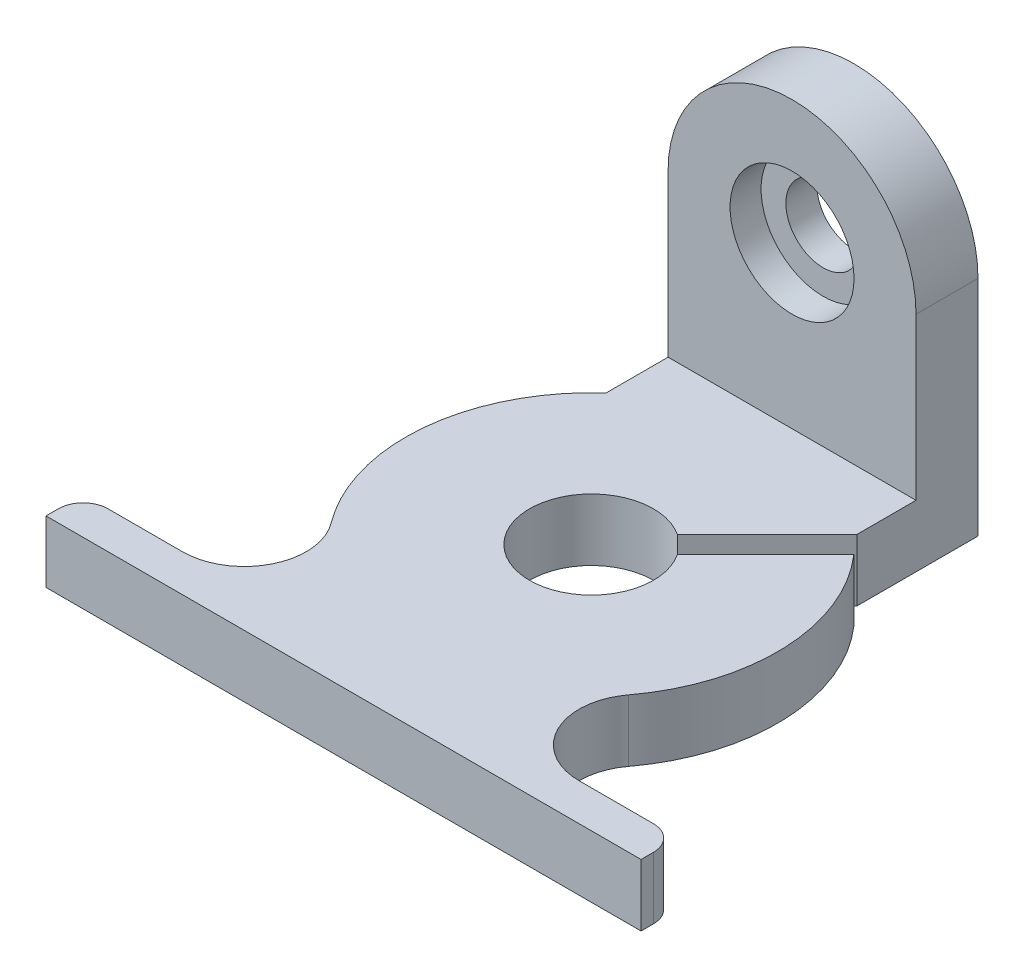
ISO-10303-21;
HEADER;
FILE_DESCRIPTION(('STEP AP214'),'2;1');
FILE_NAME('part.step','',(''),(''),'','','');
FILE_SCHEMA(('AUTOMOTIVE_DESIGN { 1 0 10303 214 1 1 1 1 }'));
ENDSEC;
DATA;
#1=APPLICATION_CONTEXT('core data for automotive mechanical design processes');
#2=APPLICATION_PROTOCOL_DEFINITION('international standard','automotive_design',2000,#1);
#3=PRODUCT_CONTEXT('',#1,'mechanical');
#4=PRODUCT('Part','Part','',(#3));
#5=PRODUCT_RELATED_PRODUCT_CATEGORY('part','',(#4));
#6=PRODUCT_DEFINITION_FORMATION('','',#4);
#7=PRODUCT_DEFINITION_CONTEXT('part definition',#1,'design');
#8=PRODUCT_DEFINITION('design','',#6,#7);
#9=PRODUCT_DEFINITION_SHAPE('','',#8);
#10=(LENGTH_UNIT() NAMED_UNIT(*) SI_UNIT(.MILLI.,.METRE.));
#11=(NAMED_UNIT(*) PLANE_ANGLE_UNIT() SI_UNIT($,.RADIAN.));
#12=(NAMED_UNIT(*) SI_UNIT($,.STERADIAN.) SOLID_ANGLE_UNIT());
#13=UNCERTAINTY_MEASURE_WITH_UNIT(LENGTH_MEASURE(1.E-05),#10,'distance_accuracy_value','');
#14=(GEOMETRIC_REPRESENTATION_CONTEXT(3) GLOBAL_UNCERTAINTY_ASSIGNED_CONTEXT((#13)) GLOBAL_UNIT_ASSIGNED_CONTEXT((#10,
#11,#12)) REPRESENTATION_CONTEXT('',''));
#15=CARTESIAN_POINT('',(0.,0.,0.));
#16=DIRECTION('',(0.,0.,1.));
#17=DIRECTION('',(1.,0.,0.));
#18=AXIS2_PLACEMENT_3D('',#15,#16,#17);
#19=CARTESIAN_POINT('',(0.,18.,-36.180339887499));
#20=DIRECTION('',(0.,0.,-1.));
#21=DIRECTION('',(-1.,0.,0.));
#22=AXIS2_PLACEMENT_3D('',#19,#20,#21);
#23=CYLINDRICAL_SURFACE('',#22,3.);
#24=CARTESIAN_POINT('',(0.,18.,-41.180339887499));
#25=DIRECTION('',(0.,0.,-1.));
#26=DIRECTION('',(-1.,0.,0.));
#27=AXIS2_PLACEMENT_3D('',#24,#25,#26);
#28=CIRCLE('',#27,3.);
#29=CARTESIAN_POINT('',(-3.,18.,-41.180339887499));
#30=VERTEX_POINT('',#29);
#31=EDGE_CURVE('E596',#30,#30,#28,.T.);
#32=ORIENTED_EDGE('',*,*,#31,.T.);
#33=EDGE_LOOP('',(#32));
#34=FACE_BOUND('',#33,.T.);
#35=CARTESIAN_POINT('',(0.,18.,-38.680339887499));
#36=DIRECTION('',(0.,0.,1.));
#37=DIRECTION('',(1.,0.,0.));
#38=AXIS2_PLACEMENT_3D('',#35,#36,#37);
#39=CIRCLE('',#38,3.);
#40=CARTESIAN_POINT('',(3.,18.,-38.680339887499));
#41=VERTEX_POINT('',#40);
#42=EDGE_CURVE('E609',#41,#41,#39,.T.);
#43=ORIENTED_EDGE('',*,*,#42,.T.);
#44=EDGE_LOOP('',(#43));
#45=FACE_BOUND('',#44,.T.);
#46=ADVANCED_FACE('F50',(#34,#45),#23,.F.);
#47=CARTESIAN_POINT('',(0.,5.,0.));
#48=DIRECTION('',(0.,1.,0.));
#49=DIRECTION('',(0.,0.,1.));
#50=AXIS2_PLACEMENT_3D('',#47,#48,#49);
#51=PLANE('',#50);
#52=DIRECTION('',(0.,0.,-1.));
#53=VECTOR('',#52,1.);
#54=CARTESIAN_POINT('',(10.,5.,0.));
#55=LINE('',#54,#53);
#56=CARTESIAN_POINT('',(10.,5.,-31.4142135623731));
#57=VERTEX_POINT('',#56);
#58=CARTESIAN_POINT('',(10.,5.,-36.180339887499));
#59=VERTEX_POINT('',#58);
#60=EDGE_CURVE('E197',#57,#59,#55,.T.);
#61=ORIENTED_EDGE('',*,*,#60,.T.);
#62=DIRECTION('',(-1.,0.,0.));
#63=VECTOR('',#62,1.);
#64=CARTESIAN_POINT('',(0.,5.,-36.180339887499));
#65=LINE('',#64,#63);
#66=CARTESIAN_POINT('',(-10.,5.,-36.180339887499));
#67=VERTEX_POINT('',#66);
#68=EDGE_CURVE('E202',#59,#67,#65,.T.);
#69=ORIENTED_EDGE('',*,*,#68,.T.);
#70=DIRECTION('',(0.,0.,-1.));
#71=VECTOR('',#70,1.);
#72=CARTESIAN_POINT('',(-10.,5.,0.));
#73=LINE('',#72,#71);
#74=CARTESIAN_POINT('',(-10.,5.,-31.1803398874989));
#75=VERTEX_POINT('',#74);
#76=EDGE_CURVE('E241',#75,#67,#73,.T.);
#77=ORIENTED_EDGE('',*,*,#76,.F.);
#78=CARTESIAN_POINT('',(0.,5.,-20.));
#79=DIRECTION('',(0.,1.,0.));
#80=DIRECTION('',(0.,0.,1.));
#81=AXIS2_PLACEMENT_3D('',#78,#79,#80);
#82=CIRCLE('',#81,15.);
#83=CARTESIAN_POINT('',(-12.,5.,-11.));
#84=VERTEX_POINT('',#83);
#85=EDGE_CURVE('E291',#75,#84,#82,.T.);
#86=ORIENTED_EDGE('',*,*,#85,.T.);
#87=CARTESIAN_POINT('',(-16.,5.,-8.));
#88=DIRECTION('',(0.,1.,0.));
#89=DIRECTION('',(0.,0.,1.));
#90=AXIS2_PLACEMENT_3D('',#87,#88,#89);
#91=CIRCLE('',#90,5.);
#92=CARTESIAN_POINT('',(-16.,5.,-3.));
#93=VERTEX_POINT('',#92);
#94=EDGE_CURVE('E280',#84,#93,#91,.F.);
#95=ORIENTED_EDGE('',*,*,#94,.T.);
#96=DIRECTION('',(1.,0.,0.));
#97=VECTOR('',#96,1.);
#98=CARTESIAN_POINT('',(0.,5.,-3.));
#99=LINE('',#98,#97);
#100=CARTESIAN_POINT('',(-22.,5.,-3.));
#101=VERTEX_POINT('',#100);
#102=EDGE_CURVE('E288',#101,#93,#99,.T.);
#103=ORIENTED_EDGE('',*,*,#102,.F.);
#104=CARTESIAN_POINT('',(-22.,5.,-1.));
#105=DIRECTION('',(0.,1.,0.));
#106=DIRECTION('',(0.,0.,1.));
#107=AXIS2_PLACEMENT_3D('',#104,#105,#106);
#108=CIRCLE('',#107,2.);
#109=CARTESIAN_POINT('',(-24.,5.,-0.999999999999985));
#110=VERTEX_POINT('',#109);
#111=EDGE_CURVE('E290',#110,#101,#108,.F.);
#112=ORIENTED_EDGE('',*,*,#111,.F.);
#113=DIRECTION('',(0.,0.,-1.));
#114=VECTOR('',#113,1.);
#115=CARTESIAN_POINT('',(-24.,5.,0.));
#116=LINE('',#115,#114);
#117=CARTESIAN_POINT('',(-24.,5.,0.));
#118=VERTEX_POINT('',#117);
#119=EDGE_CURVE('E292',#118,#110,#116,.T.);
#120=ORIENTED_EDGE('',*,*,#119,.F.);
#121=DIRECTION('',(1.,0.,0.));
#122=VECTOR('',#121,1.);
#123=CARTESIAN_POINT('',(0.,5.,0.));
#124=LINE('',#123,#122);
#125=CARTESIAN_POINT('',(24.,5.,0.));
#126=VERTEX_POINT('',#125);
#127=EDGE_CURVE('E300',#118,#126,#124,.T.);
#128=ORIENTED_EDGE('',*,*,#127,.T.);
#129=DIRECTION('',(0.,0.,1.));
#130=VECTOR('',#129,1.);
#131=CARTESIAN_POINT('',(24.,5.,0.));
#132=LINE('',#131,#130);
#133=CARTESIAN_POINT('',(24.,5.,-0.999999999999985));
#134=VERTEX_POINT('',#133);
#135=EDGE_CURVE('E303',#134,#126,#132,.T.);
#136=ORIENTED_EDGE('',*,*,#135,.F.);
#137=CARTESIAN_POINT('',(22.,5.,-1.));
#138=DIRECTION('',(0.,1.,0.));
#139=DIRECTION('',(0.,0.,1.));
#140=AXIS2_PLACEMENT_3D('',#137,#138,#139);
#141=CIRCLE('',#140,2.);
#142=CARTESIAN_POINT('',(22.,5.,-3.));
#143=VERTEX_POINT('',#142);
#144=EDGE_CURVE('E305',#143,#134,#141,.F.);
#145=ORIENTED_EDGE('',*,*,#144,.F.);
#146=DIRECTION('',(1.,0.,0.));
#147=VECTOR('',#146,1.);
#148=CARTESIAN_POINT('',(0.,5.,-3.));
#149=LINE('',#148,#147);
#150=CARTESIAN_POINT('',(16.,5.,-3.));
#151=VERTEX_POINT('',#150);
#152=EDGE_CURVE('E307',#151,#143,#149,.T.);
#153=ORIENTED_EDGE('',*,*,#152,.F.);
#154=CARTESIAN_POINT('',(16.,5.,-8.));
#155=DIRECTION('',(0.,1.,0.));
#156=DIRECTION('',(0.,0.,1.));
#157=AXIS2_PLACEMENT_3D('',#154,#155,#156);
#158=CIRCLE('',#157,5.);
#159=CARTESIAN_POINT('',(12.,5.,-11.));
#160=VERTEX_POINT('',#159);
#161=EDGE_CURVE('E309',#160,#151,#158,.T.);
#162=ORIENTED_EDGE('',*,*,#161,.F.);
#163=CARTESIAN_POINT('',(0.,5.,-20.));
#164=DIRECTION('',(0.,1.,0.));
#165=DIRECTION('',(0.,0.,1.));
#166=AXIS2_PLACEMENT_3D('',#163,#164,#165);
#167=CIRCLE('',#166,15.);
#168=CARTESIAN_POINT('',(11.2901120254449,5.,-29.8758984630718));
#169=VERTEX_POINT('',#168);
#170=EDGE_CURVE('E194',#160,#169,#167,.T.);
#171=ORIENTED_EDGE('',*,*,#170,.T.);
#172=DIRECTION('',(0.707106781186549,0.,-0.707106781186546));
#173=VECTOR('',#172,1.);
#174=CARTESIAN_POINT('',(-9.29289321881346,5.,-9.29289321881349));
#175=LINE('',#174,#173);
#176=CARTESIAN_POINT('',(4.17120839632431,5.,-22.7569948339512));
#177=VERTEX_POINT('',#176);
#178=EDGE_CURVE('E177',#177,#169,#175,.T.);
#179=ORIENTED_EDGE('',*,*,#178,.F.);
#180=CARTESIAN_POINT('',(0.,5.,-20.));
#181=DIRECTION('',(0.,1.,0.));
#182=DIRECTION('',(0.,0.,1.));
#183=AXIS2_PLACEMENT_3D('',#180,#181,#182);
#184=CIRCLE('',#183,5.);
#185=CARTESIAN_POINT('',(2.75699483395122,5.,-24.1712083963243));
#186=VERTEX_POINT('',#185);
#187=EDGE_CURVE('E190',#186,#177,#184,.T.);
#188=ORIENTED_EDGE('',*,*,#187,.F.);
#189=DIRECTION('',(0.707106781186549,0.,-0.707106781186547));
#190=VECTOR('',#189,1.);
#191=CARTESIAN_POINT('',(-10.7071067811865,5.,-10.7071067811866));
#192=LINE('',#191,#190);
#193=EDGE_CURVE('E65',#186,#57,#192,.T.);
#194=ORIENTED_EDGE('',*,*,#193,.T.);
#195=EDGE_LOOP('',(#61,#69,#77,#86,#95,#103,#112,#120,#128,#136,#145,#153,#162,#171,#179,#188,#194));
#196=FACE_BOUND('',#195,.T.);
#197=ADVANCED_FACE('F187',(#196),#51,.T.);
#198=CARTESIAN_POINT('',(-10.,5.,0.));
#199=DIRECTION('',(-1.,0.,0.));
#200=DIRECTION('',(0.,0.,1.));
#201=AXIS2_PLACEMENT_3D('',#198,#199,#200);
#202=PLANE('',#201);
#203=DIRECTION('',(0.,-1.,0.));
#204=VECTOR('',#203,1.);
#205=CARTESIAN_POINT('',(-10.,5.,-41.180339887499));
#206=LINE('',#205,#204);
#207=CARTESIAN_POINT('',(-10.,18.,-41.180339887499));
#208=VERTEX_POINT('',#207);
#209=CARTESIAN_POINT('',(-10.,0.,-41.180339887499));
#210=VERTEX_POINT('',#209);
#211=EDGE_CURVE('E205',#208,#210,#206,.T.);
#212=ORIENTED_EDGE('',*,*,#211,.T.);
#213=DIRECTION('',(0.,0.,-1.));
#214=VECTOR('',#213,1.);
#215=CARTESIAN_POINT('',(-10.,0.,0.));
#216=LINE('',#215,#214);
#217=CARTESIAN_POINT('',(-10.,0.,-31.1803398874989));
#218=VERTEX_POINT('',#217);
#219=EDGE_CURVE('E129',#218,#210,#216,.T.);
#220=ORIENTED_EDGE('',*,*,#219,.F.);
#221=DIRECTION('',(0.,-1.,0.));
#222=VECTOR('',#221,1.);
#223=CARTESIAN_POINT('',(-10.,5.,-31.1803398874989));
#224=LINE('',#223,#222);
#225=EDGE_CURVE('E11',#75,#218,#224,.T.);
#226=ORIENTED_EDGE('',*,*,#225,.F.);
#227=ORIENTED_EDGE('',*,*,#76,.T.);
#228=DIRECTION('',(0.,1.,0.));
#229=VECTOR('',#228,1.);
#230=CARTESIAN_POINT('',(-10.,0.,-36.180339887499));
#231=LINE('',#230,#229);
#232=CARTESIAN_POINT('',(-10.,18.,-36.180339887499));
#233=VERTEX_POINT('',#232);
#234=EDGE_CURVE('E589',#67,#233,#231,.T.);
#235=ORIENTED_EDGE('',*,*,#234,.T.);
#236=DIRECTION('',(0.,0.,-1.));
#237=VECTOR('',#236,1.);
#238=CARTESIAN_POINT('',(-10.,18.,-36.180339887499));
#239=LINE('',#238,#237);
#240=EDGE_CURVE('E584',#233,#208,#239,.T.);
#241=ORIENTED_EDGE('',*,*,#240,.T.);
#242=EDGE_LOOP('',(#212,#220,#226,#227,#235,#241));
#243=FACE_BOUND('',#242,.T.);
#244=ADVANCED_FACE('F47',(#243),#202,.T.);
#245=CARTESIAN_POINT('',(0.,5.,-20.));
#246=DIRECTION('',(0.,-1.,0.));
#247=DIRECTION('',(0.,0.,-1.));
#248=AXIS2_PLACEMENT_3D('',#245,#246,#247);
#249=CYLINDRICAL_SURFACE('',#248,15.);
#250=CARTESIAN_POINT('',(0.,0.,-20.));
#251=DIRECTION('',(0.,1.,0.));
#252=DIRECTION('',(0.,0.,1.));
#253=AXIS2_PLACEMENT_3D('',#250,#251,#252);
#254=CIRCLE('',#253,15.);
#255=CARTESIAN_POINT('',(-12.,0.,-11.));
#256=VERTEX_POINT('',#255);
#257=EDGE_CURVE('E204',#218,#256,#254,.T.);
#258=ORIENTED_EDGE('',*,*,#257,.T.);
#259=DIRECTION('',(0.,-1.,0.));
#260=VECTOR('',#259,1.);
#261=CARTESIAN_POINT('',(-12.,5.,-11.));
#262=LINE('',#261,#260);
#263=EDGE_CURVE('E57',#84,#256,#262,.T.);
#264=ORIENTED_EDGE('',*,*,#263,.F.);
#265=ORIENTED_EDGE('',*,*,#85,.F.);
#266=ORIENTED_EDGE('',*,*,#225,.T.);
#267=EDGE_LOOP('',(#258,#264,#265,#266));
#268=FACE_BOUND('',#267,.T.);
#269=ADVANCED_FACE('F439',(#268),#249,.T.);
#270=CARTESIAN_POINT('',(-16.,5.,-8.));
#271=DIRECTION('',(0.,-1.,0.));
#272=DIRECTION('',(0.,0.,-1.));
#273=AXIS2_PLACEMENT_3D('',#270,#271,#272);
#274=CYLINDRICAL_SURFACE('',#273,5.);
#275=CARTESIAN_POINT('',(-16.,0.,-8.));
#276=DIRECTION('',(0.,1.,0.));
#277=DIRECTION('',(0.,0.,1.));
#278=AXIS2_PLACEMENT_3D('',#275,#276,#277);
#279=CIRCLE('',#278,5.);
#280=CARTESIAN_POINT('',(-16.,0.,-3.));
#281=VERTEX_POINT('',#280);
#282=EDGE_CURVE('E210',#256,#281,#279,.F.);
#283=ORIENTED_EDGE('',*,*,#282,.T.);
#284=DIRECTION('',(0.,-1.,0.));
#285=VECTOR('',#284,1.);
#286=CARTESIAN_POINT('',(-16.,5.,-3.));
#287=LINE('',#286,#285);
#288=EDGE_CURVE('E267',#93,#281,#287,.T.);
#289=ORIENTED_EDGE('',*,*,#288,.F.);
#290=ORIENTED_EDGE('',*,*,#94,.F.);
#291=ORIENTED_EDGE('',*,*,#263,.T.);
#292=EDGE_LOOP('',(#283,#289,#290,#291));
#293=FACE_BOUND('',#292,.T.);
#294=ADVANCED_FACE('F274',(#293),#274,.F.);
#295=CARTESIAN_POINT('',(0.,5.,-3.));
#296=DIRECTION('',(0.,0.,-1.));
#297=DIRECTION('',(-1.,0.,0.));
#298=AXIS2_PLACEMENT_3D('',#295,#296,#297);
#299=PLANE('',#298);
#300=DIRECTION('',(1.,0.,0.));
#301=VECTOR('',#300,1.);
#302=CARTESIAN_POINT('',(0.,0.,-3.));
#303=LINE('',#302,#301);
#304=CARTESIAN_POINT('',(-22.,0.,-3.));
#305=VERTEX_POINT('',#304);
#306=EDGE_CURVE('E209',#305,#281,#303,.T.);
#307=ORIENTED_EDGE('',*,*,#306,.F.);
#308=DIRECTION('',(0.,-1.,0.));
#309=VECTOR('',#308,1.);
#310=CARTESIAN_POINT('',(-22.,5.,-3.));
#311=LINE('',#310,#309);
#312=EDGE_CURVE('E270',#101,#305,#311,.T.);
#313=ORIENTED_EDGE('',*,*,#312,.F.);
#314=ORIENTED_EDGE('',*,*,#102,.T.);
#315=ORIENTED_EDGE('',*,*,#288,.T.);
#316=EDGE_LOOP('',(#307,#313,#314,#315));
#317=FACE_BOUND('',#316,.T.);
#318=ADVANCED_FACE('F282',(#317),#299,.T.);
#319=CARTESIAN_POINT('',(-22.,5.,-1.));
#320=DIRECTION('',(0.,-1.,0.));
#321=DIRECTION('',(0.,0.,-1.));
#322=AXIS2_PLACEMENT_3D('',#319,#320,#321);
#323=CYLINDRICAL_SURFACE('',#322,2.);
#324=CARTESIAN_POINT('',(-22.,0.,-1.));
#325=DIRECTION('',(0.,1.,0.));
#326=DIRECTION('',(0.,0.,1.));
#327=AXIS2_PLACEMENT_3D('',#324,#325,#326);
#328=CIRCLE('',#327,2.);
#329=CARTESIAN_POINT('',(-24.,0.,-0.999999999999985));
#330=VERTEX_POINT('',#329);
#331=EDGE_CURVE('E213',#330,#305,#328,.F.);
#332=ORIENTED_EDGE('',*,*,#331,.F.);
#333=DIRECTION('',(0.,-1.,0.));
#334=VECTOR('',#333,1.);
#335=CARTESIAN_POINT('',(-24.,5.,-0.999999999999985));
#336=LINE('',#335,#334);
#337=EDGE_CURVE('E264',#110,#330,#336,.T.);
#338=ORIENTED_EDGE('',*,*,#337,.F.);
#339=ORIENTED_EDGE('',*,*,#111,.T.);
#340=ORIENTED_EDGE('',*,*,#312,.T.);
#341=EDGE_LOOP('',(#332,#338,#339,#340));
#342=FACE_BOUND('',#341,.T.);
#343=ADVANCED_FACE('F533',(#342),#323,.T.);
#344=CARTESIAN_POINT('',(-24.,5.,0.));
#345=DIRECTION('',(-1.,0.,0.));
#346=DIRECTION('',(0.,0.,1.));
#347=AXIS2_PLACEMENT_3D('',#344,#345,#346);
#348=PLANE('',#347);
#349=DIRECTION('',(0.,0.,-1.));
#350=VECTOR('',#349,1.);
#351=CARTESIAN_POINT('',(-24.,0.,0.));
#352=LINE('',#351,#350);
#353=CARTESIAN_POINT('',(-24.,0.,0.));
#354=VERTEX_POINT('',#353);
#355=EDGE_CURVE('E216',#354,#330,#352,.T.);
#356=ORIENTED_EDGE('',*,*,#355,.F.);
#357=DIRECTION('',(0.,-1.,0.));
#358=VECTOR('',#357,1.);
#359=CARTESIAN_POINT('',(-24.,5.,0.));
#360=LINE('',#359,#358);
#361=EDGE_CURVE('E263',#118,#354,#360,.T.);
#362=ORIENTED_EDGE('',*,*,#361,.F.);
#363=ORIENTED_EDGE('',*,*,#119,.T.);
#364=ORIENTED_EDGE('',*,*,#337,.T.);
#365=EDGE_LOOP('',(#356,#362,#363,#364));
#366=FACE_BOUND('',#365,.T.);
#367=ADVANCED_FACE('F523',(#366),#348,.T.);
#368=CARTESIAN_POINT('',(0.,5.,0.));
#369=DIRECTION('',(0.,0.,-1.));
#370=DIRECTION('',(-1.,0.,0.));
#371=AXIS2_PLACEMENT_3D('',#368,#369,#370);
#372=PLANE('',#371);
#373=DIRECTION('',(1.,0.,0.));
#374=VECTOR('',#373,1.);
#375=CARTESIAN_POINT('',(0.,0.,0.));
#376=LINE('',#375,#374);
#377=CARTESIAN_POINT('',(24.,0.,0.));
#378=VERTEX_POINT('',#377);
#379=EDGE_CURVE('E218',#354,#378,#376,.T.);
#380=ORIENTED_EDGE('',*,*,#379,.T.);
#381=DIRECTION('',(0.,-1.,0.));
#382=VECTOR('',#381,1.);
#383=CARTESIAN_POINT('',(24.,5.,0.));
#384=LINE('',#383,#382);
#385=EDGE_CURVE('E261',#126,#378,#384,.T.);
#386=ORIENTED_EDGE('',*,*,#385,.F.);
#387=ORIENTED_EDGE('',*,*,#127,.F.);
#388=ORIENTED_EDGE('',*,*,#361,.T.);
#389=EDGE_LOOP('',(#380,#386,#387,#388));
#390=FACE_BOUND('',#389,.T.);
#391=ADVANCED_FACE('F512',(#390),#372,.F.);
#392=CARTESIAN_POINT('',(24.,5.,0.));
#393=DIRECTION('',(1.,0.,0.));
#394=DIRECTION('',(0.,0.,-1.));
#395=AXIS2_PLACEMENT_3D('',#392,#393,#394);
#396=PLANE('',#395);
#397=DIRECTION('',(0.,0.,1.));
#398=VECTOR('',#397,1.);
#399=CARTESIAN_POINT('',(24.,0.,0.));
#400=LINE('',#399,#398);
#401=CARTESIAN_POINT('',(24.,0.,-0.999999999999985));
#402=VERTEX_POINT('',#401);
#403=EDGE_CURVE('E225',#402,#378,#400,.T.);
#404=ORIENTED_EDGE('',*,*,#403,.F.);
#405=DIRECTION('',(0.,-1.,0.));
#406=VECTOR('',#405,1.);
#407=CARTESIAN_POINT('',(24.,5.,-0.999999999999985));
#408=LINE('',#407,#406);
#409=EDGE_CURVE('E259',#134,#402,#408,.T.);
#410=ORIENTED_EDGE('',*,*,#409,.F.);
#411=ORIENTED_EDGE('',*,*,#135,.T.);
#412=ORIENTED_EDGE('',*,*,#385,.T.);
#413=EDGE_LOOP('',(#404,#410,#411,#412));
#414=FACE_BOUND('',#413,.T.);
#415=ADVANCED_FACE('F503',(#414),#396,.T.);
#416=CARTESIAN_POINT('',(22.,5.,-1.));
#417=DIRECTION('',(0.,-1.,0.));
#418=DIRECTION('',(0.,0.,-1.));
#419=AXIS2_PLACEMENT_3D('',#416,#417,#418);
#420=CYLINDRICAL_SURFACE('',#419,2.);
#421=CARTESIAN_POINT('',(22.,0.,-1.));
#422=DIRECTION('',(0.,1.,0.));
#423=DIRECTION('',(0.,0.,1.));
#424=AXIS2_PLACEMENT_3D('',#421,#422,#423);
#425=CIRCLE('',#424,2.);
#426=CARTESIAN_POINT('',(22.,0.,-3.));
#427=VERTEX_POINT('',#426);
#428=EDGE_CURVE('E223',#427,#402,#425,.F.);
#429=ORIENTED_EDGE('',*,*,#428,.F.);
#430=DIRECTION('',(0.,-1.,0.));
#431=VECTOR('',#430,1.);
#432=CARTESIAN_POINT('',(22.,5.,-3.));
#433=LINE('',#432,#431);
#434=EDGE_CURVE('E260',#143,#427,#433,.T.);
#435=ORIENTED_EDGE('',*,*,#434,.F.);
#436=ORIENTED_EDGE('',*,*,#144,.T.);
#437=ORIENTED_EDGE('',*,*,#409,.T.);
#438=EDGE_LOOP('',(#429,#435,#436,#437));
#439=FACE_BOUND('',#438,.T.);
#440=ADVANCED_FACE('F495',(#439),#420,.T.);
#441=CARTESIAN_POINT('',(0.,5.,-3.));
#442=DIRECTION('',(0.,0.,-1.));
#443=DIRECTION('',(-1.,0.,0.));
#444=AXIS2_PLACEMENT_3D('',#441,#442,#443);
#445=PLANE('',#444);
#446=DIRECTION('',(1.,0.,0.));
#447=VECTOR('',#446,1.);
#448=CARTESIAN_POINT('',(0.,0.,-3.));
#449=LINE('',#448,#447);
#450=CARTESIAN_POINT('',(16.,0.,-3.));
#451=VERTEX_POINT('',#450);
#452=EDGE_CURVE('E227',#451,#427,#449,.T.);
#453=ORIENTED_EDGE('',*,*,#452,.F.);
#454=DIRECTION('',(0.,-1.,0.));
#455=VECTOR('',#454,1.);
#456=CARTESIAN_POINT('',(16.,5.,-3.));
#457=LINE('',#456,#455);
#458=EDGE_CURVE('E254',#151,#451,#457,.T.);
#459=ORIENTED_EDGE('',*,*,#458,.F.);
#460=ORIENTED_EDGE('',*,*,#152,.T.);
#461=ORIENTED_EDGE('',*,*,#434,.T.);
#462=EDGE_LOOP('',(#453,#459,#460,#461));
#463=FACE_BOUND('',#462,.T.);
#464=ADVANCED_FACE('F319',(#463),#445,.T.);
#465=CARTESIAN_POINT('',(16.,5.,-8.));
#466=DIRECTION('',(0.,-1.,0.));
#467=DIRECTION('',(0.,0.,-1.));
#468=AXIS2_PLACEMENT_3D('',#465,#466,#467);
#469=CYLINDRICAL_SURFACE('',#468,5.);
#470=CARTESIAN_POINT('',(16.,0.,-8.));
#471=DIRECTION('',(0.,1.,0.));
#472=DIRECTION('',(0.,0.,1.));
#473=AXIS2_PLACEMENT_3D('',#470,#471,#472);
#474=CIRCLE('',#473,5.);
#475=CARTESIAN_POINT('',(12.,0.,-11.));
#476=VERTEX_POINT('',#475);
#477=EDGE_CURVE('E233',#476,#451,#474,.T.);
#478=ORIENTED_EDGE('',*,*,#477,.F.);
#479=DIRECTION('',(0.,-1.,0.));
#480=VECTOR('',#479,1.);
#481=CARTESIAN_POINT('',(12.,5.,-11.));
#482=LINE('',#481,#480);
#483=EDGE_CURVE('E251',#160,#476,#482,.T.);
#484=ORIENTED_EDGE('',*,*,#483,.F.);
#485=ORIENTED_EDGE('',*,*,#161,.T.);
#486=ORIENTED_EDGE('',*,*,#458,.T.);
#487=EDGE_LOOP('',(#478,#484,#485,#486));
#488=FACE_BOUND('',#487,.T.);
#489=ADVANCED_FACE('F314',(#488),#469,.F.);
#490=CARTESIAN_POINT('',(0.,5.,-20.));
#491=DIRECTION('',(0.,-1.,0.));
#492=DIRECTION('',(0.,0.,-1.));
#493=AXIS2_PLACEMENT_3D('',#490,#491,#492);
#494=CYLINDRICAL_SURFACE('',#493,15.);
#495=CARTESIAN_POINT('',(0.,0.,-20.));
#496=DIRECTION('',(0.,1.,0.));
#497=DIRECTION('',(0.,0.,1.));
#498=AXIS2_PLACEMENT_3D('',#495,#496,#497);
#499=CIRCLE('',#498,15.);
#500=CARTESIAN_POINT('',(11.2901120254449,0.,-29.8758984630718));
#501=VERTEX_POINT('',#500);
#502=EDGE_CURVE('E235',#476,#501,#499,.T.);
#503=ORIENTED_EDGE('',*,*,#502,.T.);
#504=DIRECTION('',(0.,-1.,0.));
#505=VECTOR('',#504,1.);
#506=CARTESIAN_POINT('',(11.2901120254449,5.,-29.8758984630718));
#507=LINE('',#506,#505);
#508=EDGE_CURVE('E183',#169,#501,#507,.T.);
#509=ORIENTED_EDGE('',*,*,#508,.F.);
#510=ORIENTED_EDGE('',*,*,#170,.F.);
#511=ORIENTED_EDGE('',*,*,#483,.T.);
#512=EDGE_LOOP('',(#503,#509,#510,#511));
#513=FACE_BOUND('',#512,.T.);
#514=ADVANCED_FACE('F322',(#513),#494,.T.);
#515=CARTESIAN_POINT('',(-9.29289321881346,5.,-9.29289321881349));
#516=DIRECTION('',(-0.707106781186546,0.,-0.707106781186549));
#517=DIRECTION('',(-0.707106781186549,0.,0.707106781186546));
#518=AXIS2_PLACEMENT_3D('',#515,#516,#517);
#519=PLANE('',#518);
#520=DIRECTION('',(0.707106781186549,0.,-0.707106781186546));
#521=VECTOR('',#520,1.);
#522=CARTESIAN_POINT('',(-9.29289321881346,0.,-9.29289321881349));
#523=LINE('',#522,#521);
#524=CARTESIAN_POINT('',(4.17120839632431,0.,-22.7569948339512));
#525=VERTEX_POINT('',#524);
#526=EDGE_CURVE('E176',#525,#501,#523,.T.);
#527=ORIENTED_EDGE('',*,*,#526,.F.);
#528=DIRECTION('',(0.,-1.,0.));
#529=VECTOR('',#528,1.);
#530=CARTESIAN_POINT('',(4.17120839632431,5.,-22.7569948339512));
#531=LINE('',#530,#529);
#532=EDGE_CURVE('E171',#177,#525,#531,.T.);
#533=ORIENTED_EDGE('',*,*,#532,.F.);
#534=ORIENTED_EDGE('',*,*,#178,.T.);
#535=ORIENTED_EDGE('',*,*,#508,.T.);
#536=EDGE_LOOP('',(#527,#533,#534,#535));
#537=FACE_BOUND('',#536,.T.);
#538=ADVANCED_FACE('F179',(#537),#519,.T.);
#539=CARTESIAN_POINT('',(0.,5.,-20.));
#540=DIRECTION('',(0.,-1.,0.));
#541=DIRECTION('',(0.,0.,-1.));
#542=AXIS2_PLACEMENT_3D('',#539,#540,#541);
#543=CYLINDRICAL_SURFACE('',#542,5.);
#544=CARTESIAN_POINT('',(0.,0.,-20.));
#545=DIRECTION('',(0.,1.,0.));
#546=DIRECTION('',(0.,0.,1.));
#547=AXIS2_PLACEMENT_3D('',#544,#545,#546);
#548=CIRCLE('',#547,5.);
#549=CARTESIAN_POINT('',(2.75699483395122,0.,-24.1712083963243));
#550=VERTEX_POINT('',#549);
#551=EDGE_CURVE('E236',#550,#525,#548,.T.);
#552=ORIENTED_EDGE('',*,*,#551,.F.);
#553=DIRECTION('',(0.,-1.,0.));
#554=VECTOR('',#553,1.);
#555=CARTESIAN_POINT('',(2.75699483395122,5.,-24.1712083963243));
#556=LINE('',#555,#554);
#557=EDGE_CURVE('E188',#186,#550,#556,.T.);
#558=ORIENTED_EDGE('',*,*,#557,.F.);
#559=ORIENTED_EDGE('',*,*,#187,.T.);
#560=ORIENTED_EDGE('',*,*,#532,.T.);
#561=EDGE_LOOP('',(#552,#558,#559,#560));
#562=FACE_BOUND('',#561,.T.);
#563=ADVANCED_FACE('F191',(#562),#543,.F.);
#564=CARTESIAN_POINT('',(-10.7071067811865,5.,-10.7071067811866));
#565=DIRECTION('',(-0.707106781186547,0.,-0.707106781186549));
#566=DIRECTION('',(-0.707106781186549,0.,0.707106781186547));
#567=AXIS2_PLACEMENT_3D('',#564,#565,#566);
#568=PLANE('',#567);
#569=DIRECTION('',(0.707106781186549,0.,-0.707106781186547));
#570=VECTOR('',#569,1.);
#571=CARTESIAN_POINT('',(-10.7071067811865,0.,-10.7071067811866));
#572=LINE('',#571,#570);
#573=CARTESIAN_POINT('',(10.,0.,-31.4142135623731));
#574=VERTEX_POINT('',#573);
#575=EDGE_CURVE('E238',#550,#574,#572,.T.);
#576=ORIENTED_EDGE('',*,*,#575,.T.);
#577=DIRECTION('',(0.,-1.,0.));
#578=VECTOR('',#577,1.);
#579=CARTESIAN_POINT('',(10.,5.,-31.4142135623731));
#580=LINE('',#579,#578);
#581=EDGE_CURVE('E250',#57,#574,#580,.T.);
#582=ORIENTED_EDGE('',*,*,#581,.F.);
#583=ORIENTED_EDGE('',*,*,#193,.F.);
#584=ORIENTED_EDGE('',*,*,#557,.T.);
#585=EDGE_LOOP('',(#576,#582,#583,#584));
#586=FACE_BOUND('',#585,.T.);
#587=ADVANCED_FACE('F365',(#586),#568,.F.);
#588=CARTESIAN_POINT('',(10.,5.,0.));
#589=DIRECTION('',(-1.,0.,0.));
#590=DIRECTION('',(0.,0.,1.));
#591=AXIS2_PLACEMENT_3D('',#588,#589,#590);
#592=PLANE('',#591);
#593=DIRECTION('',(0.,-1.,0.));
#594=VECTOR('',#593,1.);
#595=CARTESIAN_POINT('',(10.,5.,-41.180339887499));
#596=LINE('',#595,#594);
#597=CARTESIAN_POINT('',(10.,18.,-41.180339887499));
#598=VERTEX_POINT('',#597);
#599=CARTESIAN_POINT('',(10.,0.,-41.180339887499));
#600=VERTEX_POINT('',#599);
#601=EDGE_CURVE('E249',#598,#600,#596,.T.);
#602=ORIENTED_EDGE('',*,*,#601,.F.);
#603=DIRECTION('',(0.,0.,-1.));
#604=VECTOR('',#603,1.);
#605=CARTESIAN_POINT('',(10.,18.,-36.180339887499));
#606=LINE('',#605,#604);
#607=CARTESIAN_POINT('',(10.,18.,-36.180339887499));
#608=VERTEX_POINT('',#607);
#609=EDGE_CURVE('E588',#608,#598,#606,.T.);
#610=ORIENTED_EDGE('',*,*,#609,.F.);
#611=DIRECTION('',(0.,-1.,0.));
#612=VECTOR('',#611,1.);
#613=CARTESIAN_POINT('',(10.,18.,-36.180339887499));
#614=LINE('',#613,#612);
#615=EDGE_CURVE('E598',#608,#59,#614,.T.);
#616=ORIENTED_EDGE('',*,*,#615,.T.);
#617=ORIENTED_EDGE('',*,*,#60,.F.);
#618=ORIENTED_EDGE('',*,*,#581,.T.);
#619=DIRECTION('',(0.,0.,-1.));
#620=VECTOR('',#619,1.);
#621=CARTESIAN_POINT('',(10.,0.,0.));
#622=LINE('',#621,#620);
#623=EDGE_CURVE('E123',#574,#600,#622,.T.);
#624=ORIENTED_EDGE('',*,*,#623,.T.);
#625=EDGE_LOOP('',(#602,#610,#616,#617,#618,#624));
#626=FACE_BOUND('',#625,.T.);
#627=ADVANCED_FACE('F356',(#626),#592,.F.);
#628=CARTESIAN_POINT('',(0.,5.,-41.180339887499));
#629=DIRECTION('',(0.,0.,-1.));
#630=DIRECTION('',(-1.,0.,0.));
#631=AXIS2_PLACEMENT_3D('',#628,#629,#630);
#632=PLANE('',#631);
#633=DIRECTION('',(1.,0.,0.));
#634=VECTOR('',#633,1.);
#635=CARTESIAN_POINT('',(0.,0.,-41.180339887499));
#636=LINE('',#635,#634);
#637=EDGE_CURVE('E242',#210,#600,#636,.T.);
#638=ORIENTED_EDGE('',*,*,#637,.F.);
#639=ORIENTED_EDGE('',*,*,#211,.F.);
#640=CARTESIAN_POINT('',(0.,18.,-41.180339887499));
#641=DIRECTION('',(0.,0.,-1.));
#642=DIRECTION('',(-1.,0.,0.));
#643=AXIS2_PLACEMENT_3D('',#640,#641,#642);
#644=CIRCLE('',#643,10.);
#645=EDGE_CURVE('E595',#208,#598,#644,.T.);
#646=ORIENTED_EDGE('',*,*,#645,.T.);
#647=ORIENTED_EDGE('',*,*,#601,.T.);
#648=EDGE_LOOP('',(#638,#639,#646,#647));
#649=FACE_BOUND('',#648,.T.);
#650=ORIENTED_EDGE('',*,*,#31,.F.);
#651=EDGE_LOOP('',(#650));
#652=FACE_BOUND('',#651,.T.);
#653=ADVANCED_FACE('F359',(#649,#652),#632,.T.);
#654=CARTESIAN_POINT('',(0.,0.,0.));
#655=DIRECTION('',(0.,1.,0.));
#656=DIRECTION('',(0.,0.,1.));
#657=AXIS2_PLACEMENT_3D('',#654,#655,#656);
#658=PLANE('',#657);
#659=ORIENTED_EDGE('',*,*,#637,.T.);
#660=ORIENTED_EDGE('',*,*,#623,.F.);
#661=ORIENTED_EDGE('',*,*,#575,.F.);
#662=ORIENTED_EDGE('',*,*,#551,.T.);
#663=ORIENTED_EDGE('',*,*,#526,.T.);
#664=ORIENTED_EDGE('',*,*,#502,.F.);
#665=ORIENTED_EDGE('',*,*,#477,.T.);
#666=ORIENTED_EDGE('',*,*,#452,.T.);
#667=ORIENTED_EDGE('',*,*,#428,.T.);
#668=ORIENTED_EDGE('',*,*,#403,.T.);
#669=ORIENTED_EDGE('',*,*,#379,.F.);
#670=ORIENTED_EDGE('',*,*,#355,.T.);
#671=ORIENTED_EDGE('',*,*,#331,.T.);
#672=ORIENTED_EDGE('',*,*,#306,.T.);
#673=ORIENTED_EDGE('',*,*,#282,.F.);
#674=ORIENTED_EDGE('',*,*,#257,.F.);
#675=ORIENTED_EDGE('',*,*,#219,.T.);
#676=EDGE_LOOP('',(#659,#660,#661,#662,#663,#664,#665,#666,#667,#668,#669,#670,#671,#672,#673,
#674,#675));
#677=FACE_BOUND('',#676,.T.);
#678=ADVANCED_FACE('F276',(#677),#658,.F.);
#679=CARTESIAN_POINT('',(0.,18.,-36.180339887499));
#680=DIRECTION('',(0.,0.,-1.));
#681=DIRECTION('',(-1.,0.,0.));
#682=AXIS2_PLACEMENT_3D('',#679,#680,#681);
#683=CYLINDRICAL_SURFACE('',#682,10.);
#684=ORIENTED_EDGE('',*,*,#645,.F.);
#685=ORIENTED_EDGE('',*,*,#240,.F.);
#686=CARTESIAN_POINT('',(0.,18.,-36.180339887499));
#687=DIRECTION('',(0.,0.,-1.));
#688=DIRECTION('',(-1.,0.,0.));
#689=AXIS2_PLACEMENT_3D('',#686,#687,#688);
#690=CIRCLE('',#689,10.);
#691=EDGE_CURVE('E594',#233,#608,#690,.T.);
#692=ORIENTED_EDGE('',*,*,#691,.T.);
#693=ORIENTED_EDGE('',*,*,#609,.T.);
#694=EDGE_LOOP('',(#684,#685,#692,#693));
#695=FACE_BOUND('',#694,.T.);
#696=ADVANCED_FACE('F348',(#695),#683,.T.);
#697=CARTESIAN_POINT('',(0.,18.,-36.180339887499));
#698=DIRECTION('',(0.,0.,-1.));
#699=DIRECTION('',(-1.,0.,0.));
#700=AXIS2_PLACEMENT_3D('',#697,#698,#699);
#701=PLANE('',#700);
#702=CARTESIAN_POINT('',(0.,18.,-36.180339887499));
#703=DIRECTION('',(0.,0.,1.));
#704=DIRECTION('',(1.,0.,0.));
#705=AXIS2_PLACEMENT_3D('',#702,#703,#704);
#706=CIRCLE('',#705,5.);
#707=CARTESIAN_POINT('',(5.,18.,-36.180339887499));
#708=VERTEX_POINT('',#707);
#709=EDGE_CURVE('E604',#708,#708,#706,.T.);
#710=ORIENTED_EDGE('',*,*,#709,.F.);
#711=EDGE_LOOP('',(#710));
#712=FACE_BOUND('',#711,.T.);
#713=ORIENTED_EDGE('',*,*,#68,.F.);
#714=ORIENTED_EDGE('',*,*,#615,.F.);
#715=ORIENTED_EDGE('',*,*,#691,.F.);
#716=ORIENTED_EDGE('',*,*,#234,.F.);
#717=EDGE_LOOP('',(#713,#714,#715,#716));
#718=FACE_BOUND('',#717,.T.);
#719=ADVANCED_FACE('F350',(#712,#718),#701,.F.);
#720=CARTESIAN_POINT('',(0.,18.,-38.680339887499));
#721=DIRECTION('',(0.,0.,1.));
#722=DIRECTION('',(1.,0.,0.));
#723=AXIS2_PLACEMENT_3D('',#720,#721,#722);
#724=CYLINDRICAL_SURFACE('',#723,5.);
#725=CARTESIAN_POINT('',(0.,18.,-38.680339887499));
#726=DIRECTION('',(0.,0.,1.));
#727=DIRECTION('',(1.,0.,0.));
#728=AXIS2_PLACEMENT_3D('',#725,#726,#727);
#729=CIRCLE('',#728,5.);
#730=CARTESIAN_POINT('',(5.,18.,-38.680339887499));
#731=VERTEX_POINT('',#730);
#732=EDGE_CURVE('E603',#731,#731,#729,.T.);
#733=ORIENTED_EDGE('',*,*,#732,.F.);
#734=EDGE_LOOP('',(#733));
#735=FACE_BOUND('',#734,.T.);
#736=ORIENTED_EDGE('',*,*,#709,.T.);
#737=EDGE_LOOP('',(#736));
#738=FACE_BOUND('',#737,.T.);
#739=ADVANCED_FACE('F341',(#735,#738),#724,.F.);
#740=CARTESIAN_POINT('',(0.,18.,-38.680339887499));
#741=DIRECTION('',(0.,0.,1.));
#742=DIRECTION('',(1.,0.,0.));
#743=AXIS2_PLACEMENT_3D('',#740,#741,#742);
#744=PLANE('',#743);
#745=ORIENTED_EDGE('',*,*,#42,.F.);
#746=EDGE_LOOP('',(#745));
#747=FACE_BOUND('',#746,.T.);
#748=ORIENTED_EDGE('',*,*,#732,.T.);
#749=EDGE_LOOP('',(#748));
#750=FACE_BOUND('',#749,.T.);
#751=ADVANCED_FACE('F382',(#747,#750),#744,.T.);
#752=CLOSED_SHELL('',(#46,#197,#244,#269,#294,#318,#343,#367,#391,#415,#440,#464,#489,#514,#538,
#563,#587,#627,#653,#678,#696,#719,#739,#751));
#753=MANIFOLD_SOLID_BREP('B2',#752);
#754=ADVANCED_BREP_SHAPE_REPRESENTATION('',(#18,#753),#14);
#755=SHAPE_DEFINITION_REPRESENTATION(#9,#754);
ENDSEC;
END-ISO-10303-21;
